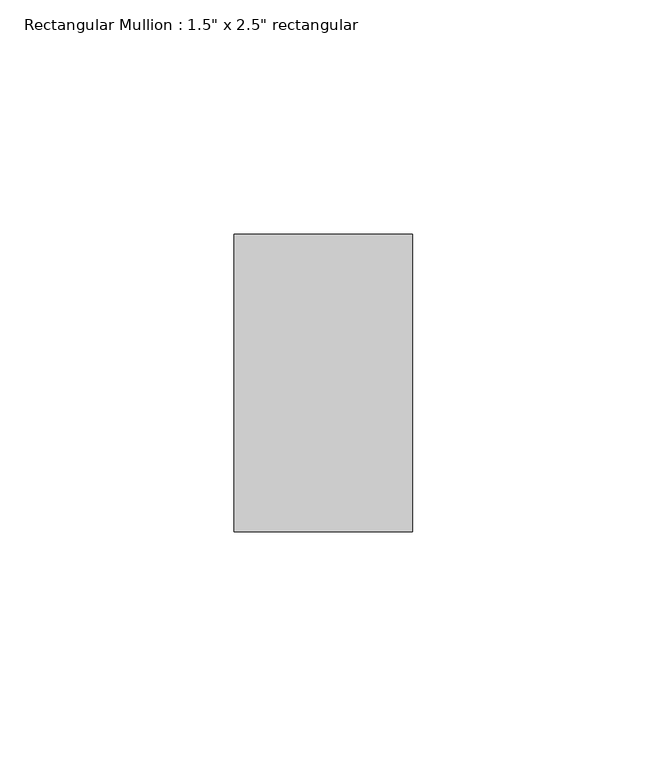
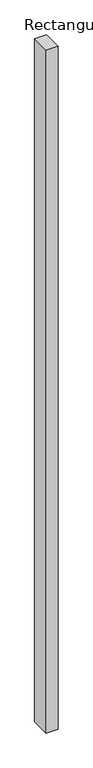
"""IFC4 building model written with IfcOpenShell, lengths in millimetres: member geometry."""

from ifc_helpers import new_model, si_unit, frame, origin, place, context, project, spatial, polyline, outline, extrude, source, transform, mapped, element, save


def member_7a5d2db7(model_context):
    return source(origin(), model_context, "Body", "SweptSolid", [
        extrude(outline(polyline([(19.05, 31.75), (19.05, -31.75), (-19.05, -31.75), (-19.05, 31.75), (19.05, 31.75)])), frame((0.0, 0.0, -2287.5875), z_axis=(0.0, 0.0, 1.0), x_axis=(1.0, 0.0, 0.0)), (0.0, 0.0, 1.0), 2287.5875),
    ])


if __name__ == "__main__":
    model = new_model("IFC4")
    model_context = context("Model", 3, world=origin())
    ifc_project = project(units=[si_unit("LENGTHUNIT", "METRE", prefix="MILLI")], contexts=[model_context])
    site = spatial("IfcSite", under=ifc_project)
    building = spatial("IfcBuilding", under=site)
    placement = place(None, origin())
    member_shape = member_7a5d2db7(model_context)
    element("IfcMember", 1, ObjectType="Rectangular Mullion : 1.5\" x 2.5\" rectangular", at=placement, inside=building, context=model_context, shape_type="MappedRepresentation", body=[
        mapped(member_shape, transform((0.0, 0.0, 0.0), x_axis=(1.0, 0.0, 0.0), y_axis=(0.0, 1.0, 0.0), z_axis=(0.0, 0.0, 1.0))),
    ])
    save(model, "model.ifc")

# Revit data of these elements
# Type "Rectangular Mullion : 1.5\" x 2.5\" rectangular"
#   built-in parameter 1007304 = 0.208333 (stored number, unit not read)
#   built-in parameter 1007301 = 0.0625 (stored number, unit not read)
#   built-in parameter 1007300 = 0.0625 (stored number, unit not read)
# Element 1 (IfcMember, "Rectangular Mullion : 1.5\" x 2.5\" rectangular")
#   Materials on its faces: "Copper"
# Materials
#   "Copper": class "Metal", colour RGB 0 0 0, transparency 0, Description = "Copper, matte finish", Cost = 0
